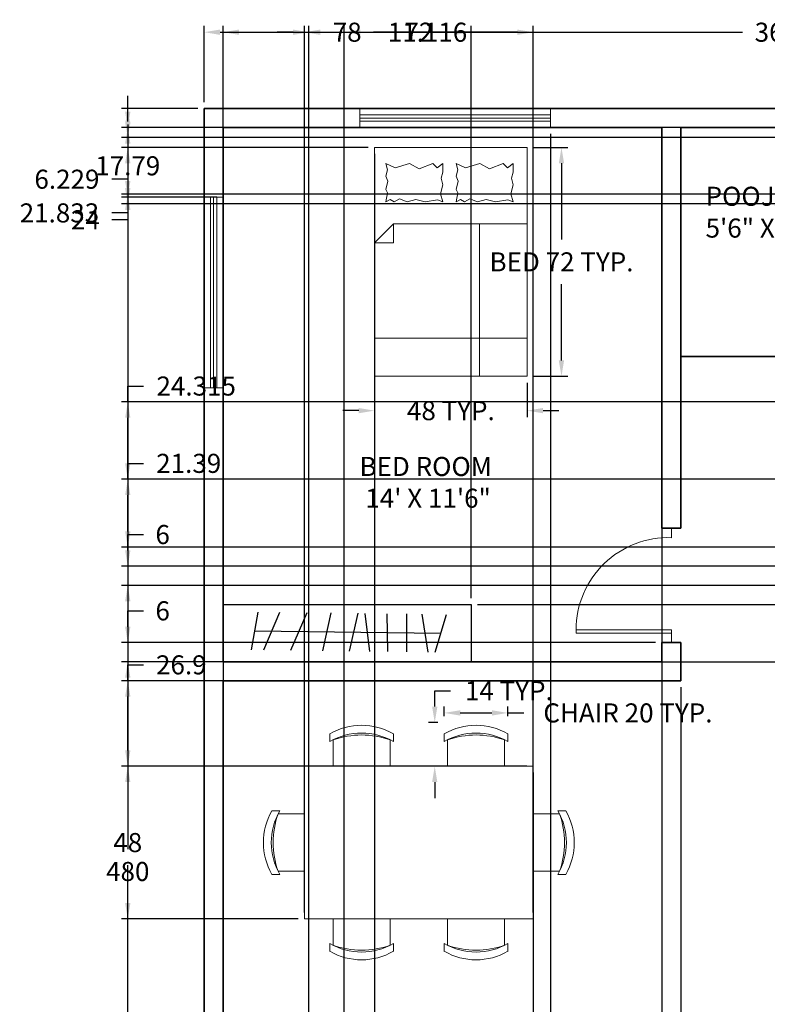
# Model space of a CAD drawing. Units: inches. Extents: x 185 to 668, y 153 to 689.
# Tile 3 of 5: x 185 to 420, y 380 to 689. Entities that reach past the tile are written whole.
import ezdxf

# ---------------------------------------------------------------- set-up
doc = ezdxf.new("R2010")
doc.units = ezdxf.units.IN
doc.header["$MEASUREMENT"] = 0
for name, color, linetype, lineweight in [('A-ANNO-DIMS', 2, 'Continuous', 18), ('A-AREA-IDEN', 7, 'Continuous', 25), ('A-DOOR', 3, 'Continuous', 18), ('A-FLOR-CASE', 8, 'Continuous', 25), ('A-FURN', 8, 'Continuous', 18), ('A-GLAZ', 4, 'Continuous', 18), ('A-WALL', 7, 'Continuous', 35)]:
    doc.layers.add(name, color=color, linetype=linetype, lineweight=lineweight)
doc.styles.get("Standard").update_dxf_attribs({"font": 'arial.ttf'})
doc.dimstyles.get("Standard").update_dxf_attribs({"dimtxt": 6, "dimasz": 5, "dimexe": 2, "dimexo": 2, "dimgap": 4, "dimtad": 0, "dimtih": 1, "dimtoh": 1, "dimdec": 0, "dimzin": 0, "dimdsep": 46, "dimlunit": 3, "dimtxsty": 'Standard', "dimcen": 2, "dimadec": 0, "dimazin": 0, "dimtfac": 1, "dimtdec": 0, "dimtofl": 0, "dimtmove": 0, "dimatfit": 3, "dimfxl": 1, "dimtolj": 1, "dimtzin": 0, "dimarcsym": 0})

# ---------------------------------------------------------------- blocks, each defined once
blk = doc.blocks.new('BED-DOUBLE-48X72')
for p, q in [((0, 72), (48, 72)), ((0, 0), (0, 72)), ((0, 72), (48, 72)), ((0, 0), (0, 72)), ((48, 72), (48, 0)), ((3.52, 66.93), (6.5, 65.56)), ((4.06, 65), (3.52, 66.93)), ((3.52, 66.93), (6.5, 65.56)), ((4.06, 65), (3.52, 66.93)), ((6.5, 65.56), (11.02, 66.93)), ((6.5, 65.56), (11.02, 66.93)), ((11.02, 66.93), (14.02, 65.28)), ((11.02, 66.93), (14.02, 65.28)), ((14.02, 65.28), (18.3, 66.93)), ((14.02, 65.28), (18.3, 66.93)), ((18.3, 66.93), (19.74, 65.6)), ((18.3, 66.93), (19.74, 65.6)), ((19.74, 65.6), (21.52, 66.93)), ((19.74, 65.6), (21.52, 66.93)), ((21.52, 66.93), (21.52, 64.24)), ((21.52, 66.93), (21.52, 64.24)), ((25.65, 66.93), (28.63, 65.56)), ((26.19, 65), (25.65, 66.93)), ((25.65, 66.93), (28.63, 65.56)), ((26.19, 65), (25.65, 66.93)), ((28.63, 65.56), (33.15, 66.93)), ((28.63, 65.56), (33.15, 66.93)), ((33.15, 66.93), (36.15, 65.28)), ((33.15, 66.93), (36.15, 65.28)), ((36.15, 65.28), (40.43, 66.93)), ((36.15, 65.28), (40.43, 66.93)), ((40.43, 66.93), (41.87, 65.6)), ((40.43, 66.93), (41.87, 65.6)), ((41.87, 65.6), (43.65, 66.93)), ((41.87, 65.6), (43.65, 66.93)), ((43.65, 66.93), (43.65, 64.24)), ((43.65, 66.93), (43.65, 64.24)), ((3.52, 63), (4.06, 65)), ((3.52, 63), (4.06, 65)), ((4.22, 61.4), (3.52, 63)), ((4.22, 61.4), (3.52, 63)), ((21.52, 64.24), (20.98, 62.32)), ((21.52, 64.24), (20.98, 62.32)), ((20.98, 62.32), (21.52, 60.2)), ((20.98, 62.32), (21.52, 60.2)), ((25.65, 63), (26.19, 65)), ((25.65, 63), (26.19, 65)), ((26.35, 61.4), (25.65, 63)), ((26.35, 61.4), (25.65, 63)), ((43.65, 64.24), (43.11, 62.32)), ((43.65, 64.24), (43.11, 62.32)), ((43.11, 62.32), (43.65, 60.2)), ((43.11, 62.32), (43.65, 60.2)), ((3.52, 58.72), (4.22, 61.4)), ((3.52, 58.72), (4.22, 61.4)), ((21.52, 60.2), (20.7, 57.36)), ((21.52, 60.2), (20.7, 57.36)), ((25.65, 58.72), (26.35, 61.4)), ((25.65, 58.72), (26.35, 61.4)), ((43.65, 60.2), (42.83, 57.36)), ((43.65, 60.2), (42.83, 57.36)), ((4.06, 57.76), (3.52, 58.72)), ((4.06, 57.76), (3.52, 58.72)), ((3.52, 54.93), (4.06, 57.76)), ((3.52, 54.93), (4.06, 57.76)), ((7.86, 55.8), (6.14, 54.93)), ((7.86, 55.8), (6.14, 54.93)), ((10.22, 54.93), (7.86, 55.8)), ((10.22, 54.93), (7.86, 55.8)), ((20.7, 57.36), (21.52, 54.93)), ((20.7, 57.36), (21.52, 54.93)), ((26.19, 57.76), (25.65, 58.72)), ((26.19, 57.76), (25.65, 58.72)), ((25.65, 54.93), (26.19, 57.76)), ((25.65, 54.93), (26.19, 57.76)), ((29.99, 55.8), (28.27, 54.93)), ((29.99, 55.8), (28.27, 54.93)), ((32.35, 54.93), (29.99, 55.8)), ((32.35, 54.93), (29.99, 55.8)), ((42.83, 57.36), (43.65, 54.93)), ((42.83, 57.36), (43.65, 54.93)), ((4.9, 55.65), (3.52, 54.93)), ((4.9, 55.65), (3.52, 54.93)), ((6.14, 54.93), (4.9, 55.65)), ((6.14, 54.93), (4.9, 55.65)), ((12.98, 55.61), (10.22, 54.93)), ((12.98, 55.61), (10.22, 54.93)), ((15.94, 54.93), (12.98, 55.61)), ((15.94, 54.93), (12.98, 55.61)), ((19.78, 55.49), (15.94, 54.93)), ((19.78, 55.49), (15.94, 54.93)), ((21.52, 54.93), (19.78, 55.49)), ((21.52, 54.93), (19.78, 55.49)), ((27.03, 55.65), (25.65, 54.93)), ((27.03, 55.65), (25.65, 54.93)), ((28.27, 54.93), (27.03, 55.65)), ((28.27, 54.93), (27.03, 55.65)), ((35.11, 55.61), (32.35, 54.93)), ((35.11, 55.61), (32.35, 54.93)), ((38.07, 54.93), (35.11, 55.61)), ((38.07, 54.93), (35.11, 55.61)), ((41.91, 55.49), (38.07, 54.93)), ((41.91, 55.49), (38.07, 54.93)), ((43.65, 54.93), (41.91, 55.49)), ((43.65, 54.93), (41.91, 55.49)), ((0, 42), (6, 48)), ((0, 42), (6, 48)), ((6, 48), (48, 48)), ((6, 48), (6, 42)), ((6, 48), (48, 48)), ((6, 48), (6, 42)), ((33, 48), (33, 0)), ((33, 48), (33, 0)), ((0, 42), (0, 0)), ((0, 42), (6, 42)), ((0, 42), (0, 0)), ((0, 42), (6, 42)), ((48, 12), (0, 12)), ((48, 12), (0, 12)), ((48, 0), (0, 0)), ((48, 0), (0, 0))]:
    blk.add_line(p, q)
blk = doc.blocks.new('CHAIR-DINING')
for p, q in [((0, 7.74), (0, 10.22)), ((20, 7.74), (20, 10.22)), ((1, 0), (1, 8.28)), ((19, 0), (19, 8.28))]:
    blk.add_line(p, q)
for centre, radius, start, end in [((10, -7.15), 20.04, 60.0663, 119.9337), ((10, -9.48), 19.92, 59.8627, 120.1373), ((10, -17.07), 26.91, 70.458, 109.542)]:
    blk.add_arc(centre, radius, start, end)
blk = doc.blocks.new('WINDOW-60')
for p, q in [((2, 60), (0, 60)), ((2, 60), (2, 0)), ((4, 60), (2, 60)), ((3, 0), (3, 60)), ((4, 0), (4, 60)), ((4, 60), (6, 60)), ((6, 0), (0, 0)), ((2, 0), (0, 0)), ((2, 0), (4, 0)), ((4, 0), (6, 0))]:
    blk.add_line(p, q)
blk = doc.blocks.new('DOOR-SINGLE-30')
for p, q in [((3, 30), (0, 30)), ((3, 30), (3, 0)), ((4, 30), (3, 30)), ((4, 0), (4, 30)), ((33, 30), (36, 30)), ((3, 0), (4, 0))]:
    blk.add_line(p, q)
blk.add_arc((4, 29.02), 29.02, 270, 1.942)
blk = doc.blocks.new('*D11')
at = {"layer": 'A-ANNO-DIMS', "color": 0, "lineweight": -2, "transparency": 16777216}
for p, q in [((318.59, 470.26), (318.59, 473.26)), ((323.59, 471.26), (333.59, 471.26)), ((338.59, 470.26), (338.59, 473.26)), ((338.59, 471.26), (343.59, 471.26))]:
    blk.add_line(p, q, dxfattribs=at)
at = {"layer": 'A-ANNO-DIMS', "color": 0, "transparency": 16777216}
for points in [[(323.59, 472.1), (323.59, 470.43), (318.59, 471.26)], [(333.59, 472.1), (333.59, 470.43), (338.59, 471.26)]]:
    blk.add_solid(points, dxfattribs=at)
at = {"layer": 'Defpoints', "color": 0, "transparency": 16777216}
for p in [(338.59, 471.26), (318.59, 468.26), (338.59, 468.26)]:
    blk.add_point(p, dxfattribs=at)
at = {"layer": 'A-ANNO-DIMS', "color": 0, "transparency": 16777216, "insert": (376.36, 471.26), "char_height": 6, "attachment_point": 5}
blk.add_mtext('\\A1;CHAIR 20 TYP.', dxfattribs=at)
blk = doc.blocks.new('*D12')
at = {"layer": 'A-ANNO-DIMS', "color": 0, "lineweight": -2, "transparency": 16777216}
for p, q in [((315.59, 473.26), (315.59, 478.26)), ((315.59, 478.26), (320.59, 478.26)), ((316.59, 468.26), (313.59, 468.26)), ((316.59, 454.48), (313.59, 454.48)), ((315.59, 449.48), (315.59, 444.48))]:
    blk.add_line(p, q, dxfattribs=at)
at = {"layer": 'A-ANNO-DIMS', "color": 0, "transparency": 16777216}
for points in [[(314.75, 473.26), (316.42, 473.26), (315.59, 468.26)], [(314.75, 449.48), (316.42, 449.48), (315.59, 454.48)]]:
    blk.add_solid(points, dxfattribs=at)
at = {"layer": 'Defpoints', "color": 0, "transparency": 16777216}
for p in [(315.59, 468.26), (318.59, 468.26), (318.59, 454.48)]:
    blk.add_point(p, dxfattribs=at)
at = {"layer": 'A-ANNO-DIMS', "color": 0, "transparency": 16777216, "insert": (338.91, 478.26), "char_height": 6, "attachment_point": 5}
blk.add_mtext('\\A1;14 TYP.', dxfattribs=at)
blk = doc.blocks.new('*D15')
at = {"layer": 'A-ANNO-DIMS', "color": 0, "lineweight": -2, "transparency": 16777216}
for p, q in [((346.66, 649.15), (357.46, 649.15)), ((355.46, 644.15), (355.46, 620.16)), ((355.46, 582.15), (355.46, 606.14)), ((346.66, 577.15), (357.46, 577.15))]:
    blk.add_line(p, q, dxfattribs=at)
at = {"layer": 'A-ANNO-DIMS', "color": 0, "transparency": 16777216}
for points in [[(354.62, 644.15), (356.29, 644.15), (355.46, 649.15)], [(354.62, 582.15), (356.29, 582.15), (355.46, 577.15)]]:
    blk.add_solid(points, dxfattribs=at)
at = {"layer": 'Defpoints', "color": 0, "transparency": 16777216}
for p in [(344.66, 649.15), (355.46, 649.15), (344.66, 577.15)]:
    blk.add_point(p, dxfattribs=at)
at = {"layer": 'A-ANNO-DIMS', "color": 0, "transparency": 16777216, "insert": (355.46, 613.15), "char_height": 6, "attachment_point": 5}
blk.add_mtext('\\A1;BED 72 TYP.', dxfattribs=at)
blk = doc.blocks.new('*D16')
at = {"layer": 'A-ANNO-DIMS', "color": 0, "lineweight": -2, "transparency": 16777216}
for p, q in [((296.66, 575.15), (296.66, 564.35)), ((344.66, 575.15), (344.66, 564.35)), ((291.66, 566.35), (286.66, 566.35)), ((349.66, 566.35), (354.66, 566.35))]:
    blk.add_line(p, q, dxfattribs=at)
at = {"layer": 'A-ANNO-DIMS', "color": 0, "transparency": 16777216}
for points in [[(291.66, 567.18), (291.66, 565.52), (296.66, 566.35)], [(349.66, 567.18), (349.66, 565.52), (344.66, 566.35)]]:
    blk.add_solid(points, dxfattribs=at)
at = {"layer": 'Defpoints', "color": 0, "transparency": 16777216}
for p in [(296.66, 577.15), (344.66, 577.15), (344.66, 566.35)]:
    blk.add_point(p, dxfattribs=at)
at = {"layer": 'A-ANNO-DIMS', "color": 0, "transparency": 16777216, "insert": (320.66, 566.35), "char_height": 6, "attachment_point": 5}
blk.add_mtext('\\A1;48 TYP.', dxfattribs=at)
blk = doc.blocks.new('*D25')
at = {"layer": 'A-ANNO-DIMS', "color": 0, "lineweight": -2, "transparency": 16777216}
for p, q in [((243.04, 663.38), (243.04, 687.4)), ((248.04, 685.4), (412.42, 685.4)), ((598.04, 685.4), (433.66, 685.4)), ((603.04, 663.38), (603.04, 687.4))]:
    blk.add_line(p, q, dxfattribs=at)
at = {"layer": 'A-ANNO-DIMS', "color": 0, "transparency": 16777216}
for points in [[(248.04, 686.23), (248.04, 684.56), (243.04, 685.4)], [(598.04, 686.23), (598.04, 684.56), (603.04, 685.4)]]:
    blk.add_solid(points, dxfattribs=at)
at = {"layer": 'Defpoints', "color": 0, "transparency": 16777216}
for p in [(603.04, 685.4), (243.04, 661.38), (603.04, 661.38)]:
    blk.add_point(p, dxfattribs=at)
at = {"layer": 'A-ANNO-DIMS', "color": 0, "transparency": 16777216, "insert": (423.04, 685.4), "char_height": 6, "attachment_point": 5}
blk.add_mtext('\\A1;360', dxfattribs=at)
blk = doc.blocks.new('*D26')
at = {"layer": 'A-ANNO-DIMS', "color": 0, "lineweight": -2, "transparency": 16777216}
for p, q in [((241.04, 661.38), (217.02, 661.38)), ((219.02, 656.38), (219.02, 428.44)), ((219.02, 186.38), (219.02, 414.32)), ((241.04, 181.38), (217.02, 181.38))]:
    blk.add_line(p, q, dxfattribs=at)
at = {"layer": 'A-ANNO-DIMS', "color": 0, "transparency": 16777216}
for points in [[(218.19, 656.38), (219.86, 656.38), (219.02, 661.38)], [(218.19, 186.38), (219.86, 186.38), (219.02, 181.38)]]:
    blk.add_solid(points, dxfattribs=at)
at = {"layer": 'Defpoints', "color": 0, "transparency": 16777216}
for p in [(219.02, 661.38), (243.04, 661.38), (243.04, 181.38)]:
    blk.add_point(p, dxfattribs=at)
at = {"layer": 'A-ANNO-DIMS', "color": 0, "transparency": 16777216, "insert": (219.02, 421.38), "char_height": 6, "attachment_point": 5}
blk.add_mtext('\\A1;480', dxfattribs=at)
blk = doc.blocks.new('*D30')
at = {"layer": 'A-ANNO-DIMS', "color": 0, "lineweight": -2, "transparency": 16777216}
for p, q in [((247.04, 655.38), (217.02, 655.38)), ((219.02, 650.38), (219.02, 638.55)), ((247.04, 633.55), (217.02, 633.55)), ((219.02, 633.55), (219.02, 628.55)), ((219.02, 628.55), (214.02, 628.55))]:
    blk.add_line(p, q, dxfattribs=at)
at = {"layer": 'A-ANNO-DIMS', "color": 0, "transparency": 16777216}
for points in [[(218.19, 650.38), (219.86, 650.38), (219.02, 655.38)], [(218.19, 638.55), (219.86, 638.55), (219.02, 633.55)]]:
    blk.add_solid(points, dxfattribs=at)
at = {"layer": 'Defpoints', "color": 0, "transparency": 16777216}
for p in [(249.04, 655.38), (219.02, 633.55), (249.04, 633.55)]:
    blk.add_point(p, dxfattribs=at)
at = {"layer": 'A-ANNO-DIMS', "color": 0, "transparency": 16777216, "insert": (197.52, 628.55), "char_height": 6, "attachment_point": 5}
blk.add_mtext('\\A1;21.833', dxfattribs=at)
blk = doc.blocks.new('*D32')
at = {"layer": 'A-ANNO-DIMS', "color": 0, "lineweight": -2, "transparency": 16777216}
for p, q in [((352.02, 653.38), (352.02, 155.36)), ((387.04, 653.38), (387.04, 155.36)), ((347.02, 157.36), (342.02, 157.36)), ((392.04, 157.36), (397.04, 157.36))]:
    blk.add_line(p, q, dxfattribs=at)
at = {"layer": 'A-ANNO-DIMS', "color": 0, "transparency": 16777216}
for points in [[(347.02, 158.19), (347.02, 156.53), (352.02, 157.36)], [(392.04, 158.19), (392.04, 156.53), (387.04, 157.36)]]:
    blk.add_solid(points, dxfattribs=at)
at = {"layer": 'Defpoints', "color": 0, "transparency": 16777216}
for p in [(352.02, 655.38), (387.04, 655.38), (387.04, 157.36)]:
    blk.add_point(p, dxfattribs=at)
at = {"layer": 'A-ANNO-DIMS', "color": 0, "transparency": 16777216, "insert": (369.53, 157.36), "char_height": 6, "attachment_point": 5}
blk.add_mtext('\\A1;35.025', dxfattribs=at)
blk = doc.blocks.new('*D40')
at = {"layer": 'A-ANNO-DIMS', "color": 0, "lineweight": -2, "transparency": 16777216}
for p, q in [((274.59, 408.48), (274.59, 687.4)), ((279.59, 685.4), (302.34, 685.4)), ((341.59, 685.4), (318.83, 685.4)), ((346.59, 408.48), (346.59, 687.4))]:
    blk.add_line(p, q, dxfattribs=at)
at = {"layer": 'A-ANNO-DIMS', "color": 0, "transparency": 16777216}
for points in [[(279.59, 686.23), (279.59, 684.56), (274.59, 685.4)], [(341.59, 686.23), (341.59, 684.56), (346.59, 685.4)]]:
    blk.add_solid(points, dxfattribs=at)
at = {"layer": 'Defpoints', "color": 0, "transparency": 16777216}
for p in [(346.59, 685.4), (274.59, 406.48), (346.59, 406.48)]:
    blk.add_point(p, dxfattribs=at)
at = {"layer": 'A-ANNO-DIMS', "color": 0, "transparency": 16777216, "insert": (310.59, 685.4), "char_height": 6, "attachment_point": 5}
blk.add_mtext('\\A1;72', dxfattribs=at)
blk = doc.blocks.new('*D41')
at = {"layer": 'A-ANNO-DIMS', "color": 0, "lineweight": -2, "transparency": 16777216}
for p, q in [((272.59, 454.48), (217.02, 454.48)), ((219.02, 449.48), (219.02, 437.54)), ((219.02, 411.48), (219.02, 423.42)), ((272.59, 406.48), (217.02, 406.48))]:
    blk.add_line(p, q, dxfattribs=at)
at = {"layer": 'A-ANNO-DIMS', "color": 0, "transparency": 16777216}
for points in [[(218.19, 449.48), (219.86, 449.48), (219.02, 454.48)], [(218.19, 411.48), (219.86, 411.48), (219.02, 406.48)]]:
    blk.add_solid(points, dxfattribs=at)
at = {"layer": 'Defpoints', "color": 0, "transparency": 16777216}
for p in [(219.02, 454.48), (274.59, 454.48), (274.59, 406.48)]:
    blk.add_point(p, dxfattribs=at)
at = {"layer": 'A-ANNO-DIMS', "color": 0, "transparency": 16777216, "insert": (219.02, 430.48), "char_height": 6, "attachment_point": 5}
blk.add_mtext('\\A1;48', dxfattribs=at)
blk = doc.blocks.new('*D42')
at = {"layer": 'A-ANNO-DIMS', "color": 0, "lineweight": -2, "transparency": 16777216}
for p, q in [((487.63, 655.38), (217.02, 655.38)), ((219.02, 650.38), (219.02, 636.38)), ((487.63, 631.38), (217.02, 631.38)), ((219.02, 631.38), (219.02, 626.38)), ((219.02, 626.38), (214.02, 626.38))]:
    blk.add_line(p, q, dxfattribs=at)
at = {"layer": 'A-ANNO-DIMS', "color": 0, "transparency": 16777216}
for points in [[(218.19, 650.38), (219.86, 650.38), (219.02, 655.38)], [(218.19, 636.38), (219.86, 636.38), (219.02, 631.38)]]:
    blk.add_solid(points, dxfattribs=at)
at = {"layer": 'Defpoints', "color": 0, "transparency": 16777216}
for p in [(489.63, 655.38), (219.02, 631.38), (489.63, 631.38)]:
    blk.add_point(p, dxfattribs=at)
at = {"layer": 'A-ANNO-DIMS', "color": 0, "transparency": 16777216, "insert": (205.69, 626.38), "char_height": 6, "attachment_point": 5}
blk.add_mtext('\\A1;24', dxfattribs=at)
blk = doc.blocks.new('*D47')
at = {"layer": 'A-ANNO-DIMS', "color": 0, "lineweight": -2, "transparency": 16777216}
for p, q in [((219.02, 522.38), (219.02, 527.38)), ((219.02, 527.38), (224.02, 527.38)), ((505.35, 517.38), (217.02, 517.38)), ((505.35, 511.38), (217.02, 511.38)), ((219.02, 506.38), (219.02, 501.38))]:
    blk.add_line(p, q, dxfattribs=at)
at = {"layer": 'A-ANNO-DIMS', "color": 0, "transparency": 16777216}
for points in [[(218.19, 522.38), (219.86, 522.38), (219.02, 517.38)], [(218.19, 506.38), (219.86, 506.38), (219.02, 511.38)]]:
    blk.add_solid(points, dxfattribs=at)
at = {"layer": 'Defpoints', "color": 0, "transparency": 16777216}
for p in [(219.02, 517.38), (507.35, 517.38), (507.35, 511.38)]:
    blk.add_point(p, dxfattribs=at)
at = {"layer": 'A-ANNO-DIMS', "color": 0, "transparency": 16777216, "insert": (230, 527.38), "char_height": 6, "attachment_point": 5}
blk.add_mtext('\\A1;6', dxfattribs=at)
blk = doc.blocks.new('*D48')
at = {"layer": 'A-ANNO-DIMS', "color": 0, "lineweight": -2, "transparency": 16777216}
for p, q in [((219.02, 498.38), (219.02, 503.38)), ((219.02, 503.38), (224.02, 503.38)), ((385.04, 493.38), (217.02, 493.38)), ((385.04, 487.38), (217.02, 487.38)), ((219.02, 482.38), (219.02, 477.38))]:
    blk.add_line(p, q, dxfattribs=at)
at = {"layer": 'A-ANNO-DIMS', "color": 0, "transparency": 16777216}
for points in [[(218.19, 498.38), (219.86, 498.38), (219.02, 493.38)], [(218.19, 482.38), (219.86, 482.38), (219.02, 487.38)]]:
    blk.add_solid(points, dxfattribs=at)
at = {"layer": 'Defpoints', "color": 0, "transparency": 16777216}
for p in [(219.02, 493.38), (387.04, 493.38), (387.04, 487.38)]:
    blk.add_point(p, dxfattribs=at)
at = {"layer": 'A-ANNO-DIMS', "color": 0, "transparency": 16777216, "insert": (230, 503.38), "char_height": 6, "attachment_point": 5}
blk.add_mtext('\\A1;6', dxfattribs=at)
blk = doc.blocks.new('*D50')
at = {"layer": 'A-ANNO-DIMS', "color": 0, "lineweight": -2, "transparency": 16777216}
for p, q in [((249.04, 507.38), (249.04, 687.4)), ((254.04, 685.4), (279.76, 685.4)), ((322.04, 685.4), (296.32, 685.4)), ((327.04, 507.38), (327.04, 687.4))]:
    blk.add_line(p, q, dxfattribs=at)
at = {"layer": 'A-ANNO-DIMS', "color": 0, "transparency": 16777216}
for points in [[(254.04, 686.23), (254.04, 684.56), (249.04, 685.4)], [(322.04, 686.23), (322.04, 684.56), (327.04, 685.4)]]:
    blk.add_solid(points, dxfattribs=at)
at = {"layer": 'Defpoints', "color": 0, "transparency": 16777216}
for p in [(327.04, 685.4), (249.04, 505.38), (327.04, 505.38)]:
    blk.add_point(p, dxfattribs=at)
at = {"layer": 'A-ANNO-DIMS', "color": 0, "transparency": 16777216, "insert": (288.04, 685.4), "char_height": 6, "attachment_point": 5}
blk.add_mtext('\\A1;78', dxfattribs=at)
blk = doc.blocks.new('*D51')
at = {"layer": 'A-ANNO-DIMS', "color": 0, "lineweight": -2, "transparency": 16777216}
for p, q in [((627.06, 510.38), (627.06, 515.38)), ((329.04, 505.38), (629.06, 505.38)), ((329.04, 487.38), (629.06, 487.38)), ((627.06, 482.38), (627.06, 477.38))]:
    blk.add_line(p, q, dxfattribs=at)
at = {"layer": 'A-ANNO-DIMS', "color": 0, "transparency": 16777216}
for points in [[(626.23, 510.38), (627.89, 510.38), (627.06, 505.38)], [(626.23, 482.38), (627.89, 482.38), (627.06, 487.38)]]:
    blk.add_solid(points, dxfattribs=at)
at = {"layer": 'Defpoints', "color": 0, "transparency": 16777216}
for p in [(327.04, 505.38), (627.06, 505.38), (327.04, 487.38)]:
    blk.add_point(p, dxfattribs=at)
at = {"layer": 'A-ANNO-DIMS', "color": 0, "transparency": 16777216, "insert": (627.06, 496.38), "char_height": 6, "attachment_point": 5}
blk.add_mtext('\\A1;18', dxfattribs=at)
blk = doc.blocks.new('*D58')
at = {"layer": 'A-ANNO-DIMS', "color": 0, "lineweight": -2, "transparency": 16777216}
for p, q in [((271.02, 685.4), (266.02, 685.4)), ((276.02, 314.15), (276.02, 687.4)), ((287.14, 303.05), (287.14, 687.4)), ((292.14, 685.4), (297.14, 685.4))]:
    blk.add_line(p, q, dxfattribs=at)
at = {"layer": 'A-ANNO-DIMS', "color": 0, "transparency": 16777216}
for points in [[(271.02, 686.23), (271.02, 684.56), (276.02, 685.4)], [(292.14, 686.23), (292.14, 684.56), (287.14, 685.4)]]:
    blk.add_solid(points, dxfattribs=at)
at = {"layer": 'Defpoints', "color": 0, "transparency": 16777216}
for p in [(287.14, 685.4), (276.02, 312.15), (287.14, 301.05)]:
    blk.add_point(p, dxfattribs=at)
at = {"layer": 'A-ANNO-DIMS', "color": 0, "transparency": 16777216, "insert": (313.31, 685.4), "char_height": 6, "attachment_point": 5}
blk.add_mtext('\\A1;11.116', dxfattribs=at)
blk = doc.blocks.new('*D63')
at = {"layer": 'A-ANNO-DIMS', "color": 0, "lineweight": -2, "transparency": 16777216}
for p, q in [((219.02, 657.26), (219.02, 662.26)), ((531.97, 652.26), (217.02, 652.26)), ((531.97, 634.47), (217.02, 634.47)), ((219.02, 629.47), (219.02, 624.47))]:
    blk.add_line(p, q, dxfattribs=at)
at = {"layer": 'A-ANNO-DIMS', "color": 0, "transparency": 16777216}
for points in [[(218.19, 657.26), (219.86, 657.26), (219.02, 652.26)], [(218.19, 629.47), (219.86, 629.47), (219.02, 634.47)]]:
    blk.add_solid(points, dxfattribs=at)
at = {"layer": 'Defpoints', "color": 0, "transparency": 16777216}
for p in [(219.02, 652.26), (533.97, 652.26), (533.97, 634.47)]:
    blk.add_point(p, dxfattribs=at)
at = {"layer": 'A-ANNO-DIMS', "color": 0, "transparency": 16777216, "insert": (219.02, 643.37), "char_height": 6, "attachment_point": 5}
blk.add_mtext('\\A1;17.79', dxfattribs=at)
blk = doc.blocks.new('*D66')
at = {"layer": 'A-ANNO-DIMS', "color": 0, "lineweight": -2, "transparency": 16777216}
for p, q in [((219.02, 569.09), (219.02, 574.09)), ((219.02, 574.09), (224.02, 574.09)), ((578.09, 569.09), (217.02, 569.09)), ((219.02, 549.77), (219.02, 564.09)), ((578.09, 544.77), (217.02, 544.77))]:
    blk.add_line(p, q, dxfattribs=at)
at = {"layer": 'A-ANNO-DIMS', "color": 0, "transparency": 16777216}
for points in [[(218.19, 564.09), (219.86, 564.09), (219.02, 569.09)], [(218.19, 549.77), (219.86, 549.77), (219.02, 544.77)]]:
    blk.add_solid(points, dxfattribs=at)
at = {"layer": 'Defpoints', "color": 0, "transparency": 16777216}
for p in [(219.02, 569.09), (580.09, 569.09), (580.09, 544.77)]:
    blk.add_point(p, dxfattribs=at)
at = {"layer": 'A-ANNO-DIMS', "color": 0, "transparency": 16777216, "insert": (240.55, 574.09), "char_height": 6, "attachment_point": 5}
blk.add_mtext('\\A1;24.315', dxfattribs=at)
blk = doc.blocks.new('*D69')
at = {"layer": 'A-ANNO-DIMS', "color": 0, "lineweight": -2, "transparency": 16777216}
for p, q in [((219.02, 544.77), (219.02, 549.77)), ((219.02, 549.77), (224.02, 549.77)), ((578.09, 544.77), (217.02, 544.77)), ((219.02, 528.38), (219.02, 539.77)), ((570.5, 523.38), (217.02, 523.38))]:
    blk.add_line(p, q, dxfattribs=at)
at = {"layer": 'A-ANNO-DIMS', "color": 0, "transparency": 16777216}
for points in [[(218.19, 539.77), (219.86, 539.77), (219.02, 544.77)], [(218.19, 528.38), (219.86, 528.38), (219.02, 523.38)]]:
    blk.add_solid(points, dxfattribs=at)
at = {"layer": 'Defpoints', "color": 0, "transparency": 16777216}
for p in [(219.02, 544.77), (580.09, 544.77), (572.5, 523.38)]:
    blk.add_point(p, dxfattribs=at)
at = {"layer": 'A-ANNO-DIMS', "color": 0, "transparency": 16777216, "insert": (238.2, 549.77), "char_height": 6, "attachment_point": 5}
blk.add_mtext('\\A1;21.39', dxfattribs=at)
blk = doc.blocks.new('*D70')
at = {"layer": 'A-ANNO-DIMS', "color": 0, "lineweight": -2, "transparency": 16777216}
for p, q in [((393.04, 479.38), (393.04, 155.36)), ((346.59, 452.48), (346.59, 155.36)), ((341.59, 157.36), (336.59, 157.36)), ((398.04, 157.36), (403.04, 157.36))]:
    blk.add_line(p, q, dxfattribs=at)
at = {"layer": 'A-ANNO-DIMS', "color": 0, "transparency": 16777216}
for points in [[(341.59, 158.19), (341.59, 156.53), (346.59, 157.36)], [(398.04, 158.19), (398.04, 156.53), (393.04, 157.36)]]:
    blk.add_solid(points, dxfattribs=at)
at = {"layer": 'Defpoints', "color": 0, "transparency": 16777216}
for p in [(393.04, 481.38), (346.59, 454.48), (393.04, 157.36)]:
    blk.add_point(p, dxfattribs=at)
at = {"layer": 'A-ANNO-DIMS', "color": 0, "transparency": 16777216, "insert": (369.81, 157.36), "char_height": 6, "attachment_point": 5}
blk.add_mtext('\\A1;46.45', dxfattribs=at)
blk = doc.blocks.new('*D71')
at = {"layer": 'A-ANNO-DIMS', "color": 0, "lineweight": -2, "transparency": 16777216}
for p, q in [((219.02, 481.38), (219.02, 486.38)), ((219.02, 486.38), (224.02, 486.38)), ((391.04, 481.38), (217.02, 481.38)), ((219.02, 459.48), (219.02, 476.38)), ((344.59, 454.48), (217.02, 454.48))]:
    blk.add_line(p, q, dxfattribs=at)
at = {"layer": 'A-ANNO-DIMS', "color": 0, "transparency": 16777216}
for points in [[(218.19, 476.38), (219.86, 476.38), (219.02, 481.38)], [(218.19, 459.48), (219.86, 459.48), (219.02, 454.48)]]:
    blk.add_solid(points, dxfattribs=at)
at = {"layer": 'Defpoints', "color": 0, "transparency": 16777216}
for p in [(219.02, 481.38), (393.04, 481.38), (346.59, 454.48)]:
    blk.add_point(p, dxfattribs=at)
at = {"layer": 'A-ANNO-DIMS', "color": 0, "transparency": 16777216, "insert": (235.87, 486.38), "char_height": 6, "attachment_point": 5}
blk.add_mtext('\\A1;26.9', dxfattribs=at)
blk = doc.blocks.new('*D72')
at = {"layer": 'A-ANNO-DIMS', "color": 0, "lineweight": -2, "transparency": 16777216}
for p, q in [((249.04, 653.38), (249.04, 155.36)), ((296.66, 647.15), (296.66, 155.36)), ((254.04, 157.36), (258.64, 157.36)), ((291.66, 157.36), (287.06, 157.36))]:
    blk.add_line(p, q, dxfattribs=at)
at = {"layer": 'A-ANNO-DIMS', "color": 0, "transparency": 16777216}
for points in [[(254.04, 158.19), (254.04, 156.53), (249.04, 157.36)], [(291.66, 158.19), (291.66, 156.53), (296.66, 157.36)]]:
    blk.add_solid(points, dxfattribs=at)
at = {"layer": 'Defpoints', "color": 0, "transparency": 16777216}
for p in [(249.04, 655.38), (296.66, 649.15), (296.66, 157.36)]:
    blk.add_point(p, dxfattribs=at)
at = {"layer": 'A-ANNO-DIMS', "color": 0, "transparency": 16777216, "insert": (272.85, 157.36), "char_height": 6, "attachment_point": 5}
blk.add_mtext('\\A1;47.62', dxfattribs=at)
blk = doc.blocks.new('*D73')
at = {"layer": 'A-ANNO-DIMS', "color": 0, "lineweight": -2, "transparency": 16777216}
for p, q in [((219.02, 660.38), (219.02, 665.38)), ((290.02, 655.38), (217.02, 655.38)), ((294.66, 649.15), (217.02, 649.15)), ((219.02, 644.15), (219.02, 639.15)), ((219.02, 639.15), (214.02, 639.15))]:
    blk.add_line(p, q, dxfattribs=at)
at = {"layer": 'A-ANNO-DIMS', "color": 0, "transparency": 16777216}
for points in [[(218.19, 660.38), (219.86, 660.38), (219.02, 655.38)], [(218.19, 644.15), (219.86, 644.15), (219.02, 649.15)]]:
    blk.add_solid(points, dxfattribs=at)
at = {"layer": 'Defpoints', "color": 0, "transparency": 16777216}
for p in [(292.02, 655.38), (219.02, 649.15), (296.66, 649.15)]:
    blk.add_point(p, dxfattribs=at)
at = {"layer": 'A-ANNO-DIMS', "color": 0, "transparency": 16777216, "insert": (199.88, 639.15), "char_height": 6, "attachment_point": 5}
blk.add_mtext('\\A1;6.229', dxfattribs=at)

msp = doc.modelspace()

# ---------------------------------------------------------------- linework, layer by layer
at = {"layer": 'A-FLOR-CASE'}
for p, q in [((249.041, 487.3789), (249.041, 505.3789)), ((249.041, 505.3789), (327.041, 505.3789)), ((327.041, 505.3789), (327.041, 487.3789)), ((259.8859, 503.0059), (257.8398, 491.1151)), ((261.8455, 491.0631), (266.8144, 502.916)), ((270.3712, 490.9526), (275.4124, 502.8045)), ((280.3608, 490.823), (283.0267, 502.7058)), ((288.7399, 490.7144), (291.4786, 502.5962)), ((293.5783, 502.569), (295.0965, 490.6319)), ((300.567, 502.4783), (300.7478, 490.5587)), ((306.676, 502.3991), (306.7005, 490.4815)), ((311.5456, 502.336), (313.3754, 490.3949)), ((315.7445, 490.3642), (319.3313, 502.235)), ((258.8629, 497.0605), (317.5379, 496.2996))]:
    msp.add_line(p, q, dxfattribs=at)
at = {"layer": 'A-FURN'}
msp.add_line((319.5866, 454.4811), (337.5866, 454.4811), dxfattribs=at)
msp.add_lwpolyline([(274.5866, 454.4811), (346.5866, 454.4811), (346.5866, 406.4811), (274.5866, 406.4811)], close=True, dxfattribs=at)
at = {"layer": 'A-WALL'}
for p, q in [((603.041, 661.3789), (243.041, 661.3789)), ((243.041, 661.3789), (243.041, 181.3789)), ((249.041, 655.3789), (249.041, 487.3789)), ((387.041, 655.3789), (249.041, 655.3789)), ((387.041, 655.3789), (387.041, 529.3789)), ((393.041, 655.3789), (393.041, 589.3789)), ((441.041, 655.3789), (393.041, 655.3789)), ((393.041, 589.3789), (393.041, 529.3789)), ((429.041, 583.3789), (393.041, 583.3789)), ((387.041, 529.3789), (393.041, 529.3789)), ((387.041, 493.3789), (393.041, 493.3789)), ((387.041, 493.3789), (387.041, 487.3789)), ((393.041, 493.3789), (393.041, 481.3789)), ((387.041, 487.3789), (249.041, 487.3789)), ((393.041, 481.3789), (249.041, 481.3789)), ((249.041, 481.3789), (249.041, 265.3789))]:
    msp.add_line(p, q, dxfattribs=at)

# ---------------------------------------------------------------- block references
at = {"layer": 'A-DOOR', "extrusion": (0, 0, -1), "zscale": -1, "rotation": 90.00000000000038}
msp.add_blockref('DOOR-SINGLE-30', (-360.041, 493.379), dxfattribs=at)
at = {"layer": 'A-FURN'}
for name, p in [('BED-DOUBLE-48X72', (296.658, 577.15)), ('CHAIR-DINING', (282.587, 454.481)), ('CHAIR-DINING', (318.587, 454.481))]:
    msp.add_blockref(name, p, dxfattribs=at)
for p, rotation in [((274.5867, 420.4815), 89.9999999999985), ((346.5865, 440.4807), 269.9999999999983), ((302.5861, 406.4812), 180), ((338.5861, 406.4812), 180)]:
    msp.add_blockref('CHAIR-DINING', p, dxfattribs=dict(at, rotation=rotation))
at = {"layer": 'A-GLAZ'}
for p, rotation in [((292.0166, 661.3789), 270), ((249.0409, 633.5459), 180)]:
    msp.add_blockref('WINDOW-60', p, dxfattribs=dict(at, rotation=rotation))

# ---------------------------------------------------------------- texts
at = {"layer": 'A-AREA-IDEN', "char_height": 6, "attachment_point": 1}
for s, insert in [('POOJA\\P5\'6" X 4\'', (400.7984, 636.7874)), ('BED ROOM\\P 14\' X 11\'6"', (291.9143, 551.7897))]:
    msp.add_mtext_dynamic_manual_height_columns(s, width=69.605686, gutter_width=1, heights=[0], dxfattribs=dict(at, insert=insert))

# ---------------------------------------------------------------- dimensions: what is measured, and where the dimension line sits
at = {"layer": 'A-ANNO-DIMS'}
for base, p1, p2, override, picture, middle in [((603.041, 685.3964), (243.041, 661.3789), (603.041, 661.3789), {"dimdec": 0, "dimlfac": 1, "dimrnd": 0, "dimzin": 0, "dimdsep": 46, "dimlunit": 2}, '*D25', (423.041, 685.3964)), ((327.041, 685.3964), (249.041, 505.3789), (327.041, 505.3789), {"dimdec": 0, "dimlfac": 1, "dimrnd": 0, "dimzin": 0, "dimdsep": 46, "dimlunit": 2}, '*D50', (288.041, 685.3964)), ((287.13651, 685.39645), (276.02002, 312.14814), (287.13651, 301.05349), {"dimdec": 3, "dimlfac": 1, "dimrnd": 0, "dimzin": 0, "dimdsep": 46, "dimlunit": 2}, '*D58', (313.30636, 685.39645)), ((346.5866, 685.3964), (274.5866, 406.4811), (346.5866, 406.4811), {"dimdec": 0, "dimlfac": 1, "dimrnd": 0, "dimzin": 0, "dimdsep": 46, "dimlunit": 2}, '*D40', (310.5866, 685.3964)), ((296.6583, 157.3614), (249.041, 655.3789), (296.6583, 649.1496), {"dimdec": 2, "dimlfac": 1, "dimrnd": 0, "dimzin": 0, "dimdsep": 46, "dimlunit": 2}, '*D72', (272.8496, 157.3614)), ((387.041, 157.3614), (352.0164, 655.3789), (387.041, 655.3789), {"dimdec": 3, "dimlfac": 1, "dimrnd": 0, "dimzin": 0, "dimdsep": 46, "dimlunit": 2}, '*D32', (369.5287, 157.3614)), ((393.041, 157.3614), (346.5866, 454.4811), (393.041, 481.3789), {"dimdec": 2, "dimlfac": 1, "dimrnd": 0, "dimzin": 0, "dimdsep": 46, "dimlunit": 2}, '*D70', (369.8138, 157.3614))]:
    dim = msp.add_linear_dim(base=base, p1=p1, p2=p2, dimstyle='Standard', override=override, dxfattribs=at)
    dim.commit()
    dim.dimension.update_dxf_attribs({"geometry": picture, "text_midpoint": middle})
for base, p1, p2, override, picture, middle in [((219.0235, 649.1496), (292.0164, 655.3789), (296.6583, 649.1496), {"dimdec": 3, "dimlfac": 1, "dimrnd": 0, "dimzin": 0, "dimdsep": 46, "dimlunit": 2}, '*D73', (199.8775, 639.1496)), ((219.0235, 652.262), (533.9695, 634.4736), (533.9695, 652.262), {"dimdec": 2, "dimlfac": 1, "dimrnd": 0, "dimzin": 0, "dimdsep": 46, "dimlunit": 2}, '*D63', (219.0235, 643.3678)), ((219.0235, 661.3789), (243.041, 181.3789), (243.041, 661.3789), {"dimdec": 0, "dimlfac": 1, "dimrnd": 0, "dimzin": 0, "dimdsep": 46, "dimlunit": 2}, '*D26', (219.0235, 421.3789)), ((219.0235, 633.5461), (249.041, 655.3789), (249.041, 633.5461), {"dimdec": 3, "dimlfac": 1, "dimrnd": 0, "dimzin": 0, "dimdsep": 46, "dimlunit": 2}, '*D30', (197.518, 628.5461)), ((219.0235, 631.3789), (489.6328, 655.3789), (489.6328, 631.3789), {"dimdec": 0, "dimlfac": 1, "dimrnd": 0, "dimzin": 0, "dimdsep": 46, "dimlunit": 2}, '*D42', (205.6872, 626.3789)), ((219.0235, 569.0859), (580.0867, 544.7709), (580.0867, 569.0859), {"dimdec": 3, "dimlfac": 1, "dimrnd": 0, "dimzin": 0, "dimdsep": 46, "dimlunit": 2}, '*D66', (240.5514, 574.0859)), ((219.0235, 544.7709), (572.4952, 523.3789), (580.0867, 544.7709), {"dimdec": 2, "dimlfac": 1, "dimrnd": 0, "dimzin": 0, "dimdsep": 46, "dimlunit": 2}, '*D69', (238.2042, 549.7709)), ((219.0235, 517.3789), (507.3502, 511.3789), (507.3502, 517.3789), {"dimdec": 0, "dimlfac": 1, "dimrnd": 0, "dimzin": 0, "dimdsep": 46, "dimlunit": 2}, '*D47', (230.0044, 527.3789)), ((627.0585, 505.3789), (327.041, 487.3789), (327.041, 505.3789), {"dimdec": 0, "dimlfac": 1, "dimrnd": 0, "dimzin": 0, "dimdsep": 46, "dimlunit": 2}, '*D51', (627.0585, 496.3789)), ((219.0235, 493.3789), (387.041, 487.3789), (387.041, 493.3789), {"dimdec": 0, "dimlfac": 1, "dimrnd": 0, "dimzin": 0, "dimdsep": 46, "dimlunit": 2}, '*D48', (230.0044, 503.3789)), ((219.0235, 481.3789), (346.5866, 454.4811), (393.041, 481.3789), {"dimdec": 1, "dimlfac": 1, "dimrnd": 0, "dimzin": 0, "dimdsep": 46, "dimlunit": 2}, '*D71', (235.8734, 486.3789)), ((219.0235, 454.4811), (274.5866, 406.4811), (274.5866, 454.4811), {"dimdec": 0, "dimlfac": 1, "dimrnd": 0, "dimzin": 0, "dimdsep": 46, "dimlunit": 2}, '*D41', (219.0235, 430.4811))]:
    dim = msp.add_linear_dim(base=base, p1=p1, p2=p2, angle=90, dimstyle='Standard', override=override, dxfattribs=at)
    dim.commit()
    dim.dimension.update_dxf_attribs({"geometry": picture, "text_midpoint": middle})
for base, p1, p2, text, picture, middle in [((355.4583, 649.1496), (344.6583, 577.1496), (344.6583, 649.1496), 'BED <> TYP.', '*D15', (355.4583, 613.1496)), ((315.5866, 468.2623), (318.5866, 454.4811), (318.5866, 468.2623), '<> TYP.', '*D12', (338.9072, 478.2623))]:
    dim = msp.add_linear_dim(base=base, p1=p1, p2=p2, angle=90, text=text, dimstyle='Standard', override={"dimdec": 0, "dimlfac": 1, "dimrnd": 0, "dimzin": 0, "dimdsep": 46, "dimlunit": 2}, dxfattribs=at)
    dim.commit()
    dim.dimension.update_dxf_attribs({"geometry": picture, "text_midpoint": middle})
for base, p1, p2, text, picture, middle in [((344.6583, 566.3496), (296.6583, 577.1496), (344.6583, 577.1496), '<> TYP.', '*D16', (320.6583, 566.3496)), ((338.5866, 471.2623), (318.5866, 468.2623), (338.5866, 468.2623), 'CHAIR <> TYP.', '*D11', (376.3587, 471.2623))]:
    dim = msp.add_linear_dim(base=base, p1=p1, p2=p2, text=text, dimstyle='Standard', override={"dimdec": 0, "dimlfac": 1, "dimrnd": 0, "dimzin": 0, "dimdsep": 46, "dimlunit": 2}, dxfattribs=at)
    dim.commit()
    dim.dimension.update_dxf_attribs({"geometry": picture, "text_midpoint": middle})

doc.saveas('drawing.dxf')
